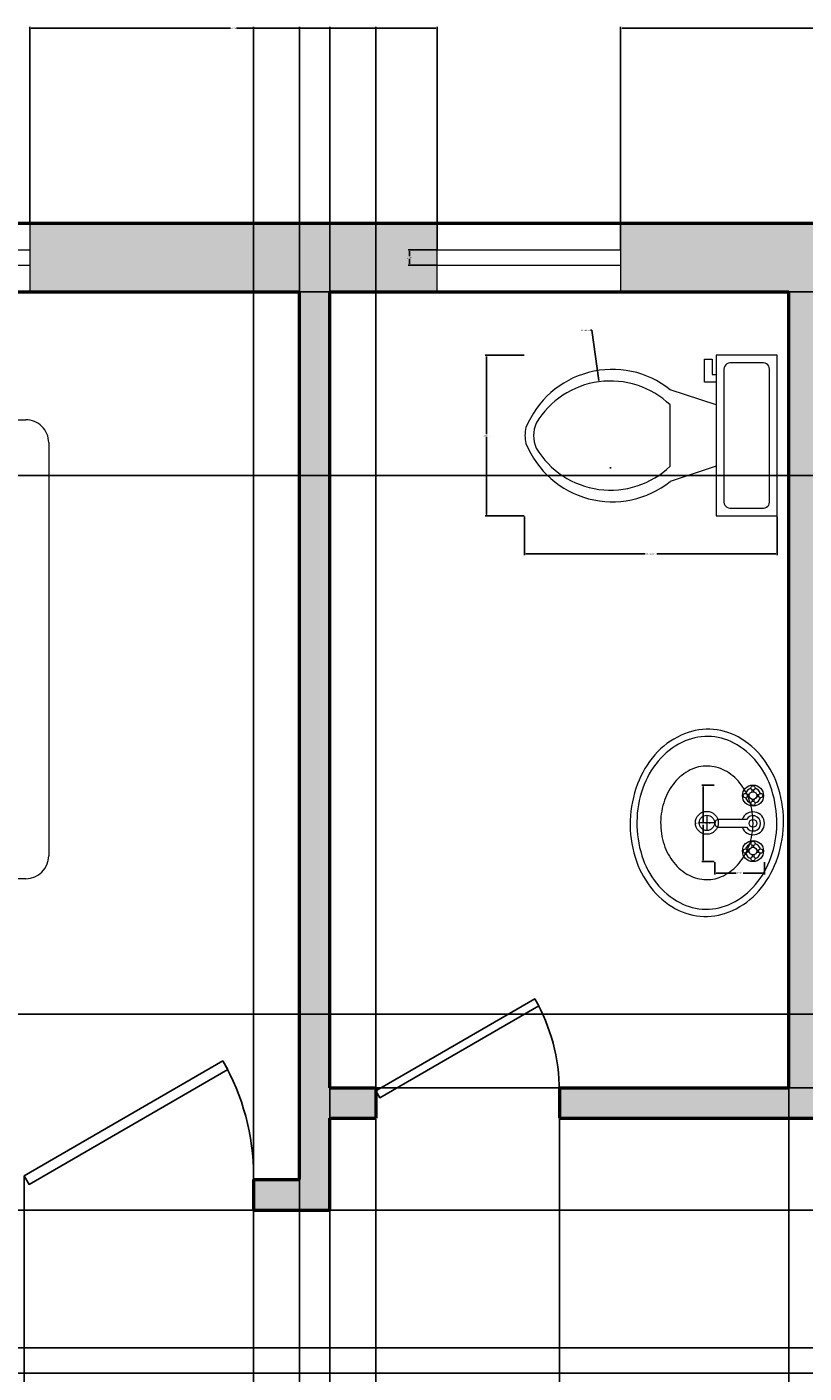
# Model space of a CAD drawing. Units: inches. Extents: x 3439 to 3988, y 1915 to 2284.
# Tile 3 of 7: x 3554 to 3656, y 2108 to 2284. Entities that reach past the tile are written whole.
import ezdxf

# ---------------------------------------------------------------- set-up
doc = ezdxf.new("R2010")
doc.units = ezdxf.units.IN
for name, color, linetype, lineweight in [('A-ANNO-DIMS', 2, 'Continuous', 18), ('A-DOOR', 3, 'Continuous', 25), ('A-FLOR-FIXT', 9, 'Continuous', 18), ('A-FURN', 9, 'Continuous', 18), ('A-GLAZ', 4, 'Continuous', 18), ('A-WALL', 7, 'Continuous', 50)]:
    doc.layers.add(name, color=color, linetype=linetype, lineweight=lineweight)
doc.layers.add('A-WALL-PATT', color=18, linetype='Continuous', lineweight=13, true_color=0x000000)
doc.styles.get("Standard").update_dxf_attribs({"font": 'arial.ttf'})
doc.dimstyles.get("Standard").update_dxf_attribs({"dimtxt": 0.18, "dimasz": 0.18, "dimexe": 0.18, "dimexo": 0.0625, "dimgap": 0.09, "dimtad": 0, "dimtih": 1, "dimtoh": 1, "dimdec": 4, "dimzin": 0, "dimdsep": 46, "dimtxsty": 'Standard', "dimcen": 0.09, "dimadec": 0, "dimazin": 0, "dimtfac": 1, "dimtdec": 4, "dimtofl": 0, "dimtmove": 0, "dimatfit": 3, "dimfxl": 1, "dimtolj": 1, "dimtzin": 0, "dimarcsym": 0})

# ---------------------------------------------------------------- blocks, each defined once
blk = doc.blocks.new('*U4')
for p, q in [((0, 0), (0, -6)), ((40, 0), (40, -6))]:
    blk.add_line(p, q)
blk.add_lwpolyline([(0, 0), (34.64, 20), (35.52, 18.48), (0.87, -1.52)], close=True)
blk.add_arc((0, 0), 40, 0, 30)
blk = doc.blocks.new('Sink - Oval top')
for p, q in [((-1, 0), (1, 0)), ((0, 1), (0, -1))]:
    blk.add_line(p, q)
for points in [[(-12.23, 0.39, 0.117634), (-11.46, -3.36, 0.104469), (-8.88, -6.8, 0.090016), (-5.08, -9.07, 0.08192), (-0.32, -10.02, 0.08192), (4.49, -9.38, 0.090016), (8.42, -7.36, 0.104469), (11.22, -4.09, 0.117634), (12.23, -0.39, 0.117634), (11.46, 3.36, 0.104469), (8.88, 6.8, 0.090016), (5.08, 9.07, 0.08192), (0.32, 10.02, 0.08192), (-4.49, 9.38, 0.090016), (-8.42, 7.36, 0.104469), (-11.22, 4.09, 0.117634)], [(-11.29, 0.16, 0.118622), (-10.52, -3.25, 0.104678), (-8.07, -6.36, 0.089562), (-4.54, -8.37, 0.081185), (-0.13, -9.15, 0.081185), (4.3, -8.49, 0.089562), (7.89, -6.58, 0.104678), (10.42, -3.55, 0.118622), (11.29, -0.16, 0.118622), (10.52, 3.25, 0.104678), (8.07, 6.36, 0.089562), (4.54, 8.37, 0.081185), (0.13, 9.15, 0.081185), (-4.3, 8.49, 0.089562), (-7.89, 6.58, 0.104678), (-10.42, 3.55, 0.118622)], [(-7.42, 0.08, 0.118283), (-6.91, -2.17, 0.104607), (-5.29, -4.21, 0.089718), (-2.97, -5.53, 0.081436), (-0.07, -6.04, 0.081436), (2.84, -5.59, 0.089718), (5.2, -4.33, 0.104607), (6.86, -2.32, 0.118283), (7.42, -0.08, 0.118283), (6.91, 2.17, 0.104607), (5.29, 4.21, 0.089718), (2.97, 5.53, 0.081436), (0.07, 6.04, 0.081436), (-2.84, 5.59, 0.089718), (-5.2, 4.33, 0.104607), (-6.86, 2.32, 0.118283)]]:
    blk.add_lwpolyline(points, format="xyb", close=True)
for radius in [1.5, 1]:
    blk.add_circle((0, 0), radius)
blk = doc.blocks.new('Faucet - Bathroom top')
for p, q in [((-4.107, 0.125), (-4.375, 0.125)), ((-3.75, 0.4788), (-3.75, 0.75)), ((-3.5, 0.482), (-3.5, 0.75)), ((-3.1461, 0.125), (-2.875, 0.125)), ((3.143, 0.125), (2.875, 0.125)), ((3.5, 0.4788), (3.5, 0.75)), ((3.75, 0.482), (3.75, 0.75)), ((4.1039, 0.125), (4.375, 0.125)), ((-4.1039, -0.125), (-4.375, -0.125)), ((-3.75, -0.4821), (-3.75, -0.75)), ((-3.5, -0.4789), (-3.5, -0.75)), ((-3.143, -0.125), (-2.875, -0.125)), ((-0.5, -0.8639), (-0.5, -4.5)), ((0.5, -4.5), (0.5, -0.8631)), ((3.1461, -0.125), (2.875, -0.125)), ((3.5, -0.4821), (3.5, -0.75)), ((3.75, -0.4789), (3.75, -0.75)), ((4.107, -0.125), (4.375, -0.125))]:
    blk.add_line(p, q)
for centre, radius in [((-3.625, 0), 1.375), ((-4.625, 0), 0.2795), ((-3.625, 0), 0.5), ((-3.625, 1), 0.2795), ((-2.625, 0), 0.2795), ((0, 0), 0.5), ((3.625, 0), 1.375), ((2.625, 0), 0.2795), ((3.625, 0), 0.5), ((3.625, 1), 0.2795), ((4.625, 0), 0.2795), ((-3.625, -1), 0.2795), ((3.625, -1), 0.2795)]:
    blk.add_circle(centre, radius)
for centre, radius, start, end in [((-3.625, 0), 1, 105.2407, 164.2093), ((-3.625, 0), 1, 16.44125, 74.07887), ((0, 0), 1.5, 289.6514, 250.3603), ((0, 0), 1, 300.3431, 239.7554), ((3.625, 0), 1, 106.12, 164.0884), ((3.625, 0), 1, 16.23422, 73.90469), ((-3.625, 0), 1, 196.2342, 253.9047), ((-3.625, 0), 1, 286.12, 344.0884), ((3.625, 0), 1, 196.4413, 254.0789), ((3.625, 0), 1, 285.2407, 344.2093), ((0, -4.5), 0.5, 180, 0)]:
    blk.add_arc(centre, radius, start, end)
blk = doc.blocks.new('Bed - Queen')
for p, q in [((3, 0), (56.99999, 0)), ((10.99999, -1.2), (25.79998, -1.2)), ((34.19999, -1.2), (48.99999, -1.2)), ((0, -77.00003), (0, -3)), ((59.99999, -3), (59.99999, -77.00003)), ((7.99999, -14.4), (7.99999, -4.2)), ((28.79998, -4.2), (28.79998, -14.4)), ((31.19999, -14.4), (31.19999, -4.2)), ((51.99999, -4.2), (51.99999, -13.4)), ((0, -14.4), (44.8, -14.4)), ((59.99999, -29.6), (44.8, -14.4)), ((44.8, -14.4), (44.8, -26.6)), ((44.8, -16.8), (0, -16.8)), ((48.99999, -16.4), (46.79936, -16.4)), ((47.8, -29.6), (59.99999, -29.6)), ((56.99999, -80.00003), (3, -80.00003))]:
    blk.add_line(p, q)
for centre, start, end in [((3, -3), 90, 180), ((56.99999, -3), 0, 90), ((10.99999, -4.2), 90, 180), ((25.79998, -4.2), 0, 90), ((34.19999, -4.2), 90, 180), ((48.99999, -4.2), 0, 90), ((48.99999, -13.4), 270, 0), ((47.8, -26.6), 180, 270), ((3, -77.00003), 180, 270), ((56.99999, -77.00003), 270, 0)]:
    blk.add_arc(centre, 3, start, end)
blk = doc.blocks.new('Toilet - top')
for p, q in [((9.5, -6), (9.5, -2)), ((-10, -8.5), (-8, -8.5)), ((-10, -9.5), (-10, -8.5)), ((-8, -8.5), (-8, -8)), ((-7, -8), (-7, -9.5)), ((-4, -8), (-6, -14)), ((4, -8), (6, -14)), ((-7, -9.5), (-10, -9.5)), ((4, -14), (-4, -14))]:
    blk.add_line(p, q)
blk.add_lwpolyline([(10.5, -8), (10.5, 0), (-10.5, 0), (-10.5, -8)], close=True)
for points in [[(8.5, -1), (-8.5, -1)], [(-9.5, -2), (-9.5, -6)], [(-8.5, -7), (8.5, -7)]]:
    blk.add_lwpolyline(points)
for centre, radius, start, end in [((-8.62, -1.88), 0.884, 81.8699, 188.1301), ((8.62, -1.88), 0.884, 351.8699, 98.1301), ((-8.62, -6.12), 0.884, 171.8699, 278.1301), ((8.62, -6.12), 0.884, 261.8699, 8.1301), ((3.52, -21.58), 12.17, 141.4691, 247.9714), ((4.2, -21.82), 11.33, 136.3677, 238.9468), ((-3.52, -21.58), 12.17, 292.0284, 38.5307), ((-4.2, -21.82), 11.33, 301.053, 43.6321), ((0, -27.88), 4, 245.7318, 294.2682), ((0, -29), 4, 254.8605, 285.1395)]:
    blk.add_arc(centre, radius, start, end)
blk = doc.blocks.new('WINDOW-GLASS-48IN')
for p, q in [((0, 2), (48, 2)), ((0, 0), (48, 0))]:
    blk.add_line(p, q)
blk = doc.blocks.new('WINDOW-GLASS-24IN')
for p, q in [((0, 2), (24, 2)), ((0, 0), (24, 0))]:
    blk.add_line(p, q)
blk = doc.blocks.new('*D21')
at = {"layer": 'A-ANNO-DIMS', "color": 0, "lineweight": -2, "transparency": 16777216}
for p, q in [((3607.59, 2254.92), (3607.59, 2258.64)), ((3607.77, 2258.46), (3618.48, 2258.46)), ((3631.41, 2258.46), (3620.71, 2258.46)), ((3631.59, 2254.92), (3631.59, 2258.64))]:
    blk.add_line(p, q, dxfattribs=at)
at = {"layer": 'A-ANNO-DIMS', "color": 0, "transparency": 16777216}
for points in [[(3607.77, 2258.49), (3607.77, 2258.43), (3607.59, 2258.46)], [(3631.41, 2258.49), (3631.41, 2258.43), (3631.59, 2258.46)]]:
    blk.add_solid(points, dxfattribs=at)
at = {"layer": 'Defpoints', "color": 0, "transparency": 16777216}
for p in [(3631.59, 2258.46), (3607.59, 2254.86), (3631.59, 2254.86)]:
    blk.add_point(p, dxfattribs=at)
at = {"layer": 'A-ANNO-DIMS', "color": 0, "transparency": 16777216, "insert": (3619.59, 2258.46), "char_height": 0.18, "attachment_point": 5}
blk.add_mtext('\\A1;WINDOW 24 TYP.', dxfattribs=at)
blk = doc.blocks.new('*D22')
at = {"layer": 'A-ANNO-DIMS', "color": 0, "lineweight": -2, "transparency": 16777216}
for p, q in [((3607.53, 2254.86), (3603.81, 2254.86)), ((3603.99, 2254.68), (3603.99, 2254.04)), ((3607.53, 2252.86), (3603.81, 2252.86)), ((3603.99, 2253.04), (3603.99, 2253.68))]:
    blk.add_line(p, q, dxfattribs=at)
at = {"layer": 'A-ANNO-DIMS', "color": 0, "transparency": 16777216}
for points in [[(3603.96, 2254.68), (3604.02, 2254.68), (3603.99, 2254.86)], [(3603.96, 2253.04), (3604.02, 2253.04), (3603.99, 2252.86)]]:
    blk.add_solid(points, dxfattribs=at)
at = {"layer": 'Defpoints', "color": 0, "transparency": 16777216}
for p in [(3603.99, 2254.86), (3607.59, 2254.86), (3607.59, 2252.86)]:
    blk.add_point(p, dxfattribs=at)
at = {"layer": 'A-ANNO-DIMS', "color": 0, "transparency": 16777216, "insert": (3603.99, 2253.86), "char_height": 0.18, "attachment_point": 5}
blk.add_mtext('\\A1;2 TYP.', dxfattribs=at)
blk = doc.blocks.new('*D31')
at = {"layer": 'A-ANNO-DIMS', "color": 0, "lineweight": -2, "transparency": 16777216}
for p, q in [((3619.03, 2220.03), (3619.03, 2214.95)), ((3652.08, 2220.03), (3652.08, 2214.95)), ((3619.21, 2215.13), (3634.78, 2215.13)), ((3651.9, 2215.13), (3636.33, 2215.13))]:
    blk.add_line(p, q, dxfattribs=at)
at = {"layer": 'A-ANNO-DIMS', "color": 0, "transparency": 16777216}
for points in [[(3619.21, 2215.16), (3619.21, 2215.1), (3619.03, 2215.13)], [(3651.9, 2215.16), (3651.9, 2215.1), (3652.08, 2215.13)]]:
    blk.add_solid(points, dxfattribs=at)
at = {"layer": 'Defpoints', "color": 0, "transparency": 16777216}
for p in [(3619.03, 2220.09), (3652.08, 2220.09), (3652.08, 2215.13)]:
    blk.add_point(p, dxfattribs=at)
at = {"layer": 'A-ANNO-DIMS', "color": 0, "transparency": 16777216, "insert": (3635.55, 2215.13), "char_height": 0.18, "attachment_point": 5}
blk.add_mtext('\\A1;WC 33 TYP.', dxfattribs=at)
blk = doc.blocks.new('*D32')
at = {"layer": 'A-ANNO-DIMS', "color": 0, "lineweight": -2, "transparency": 16777216}
for p, q in [((3618.97, 2241.09), (3613.89, 2241.09)), ((3614.07, 2240.91), (3614.07, 2230.77)), ((3614.07, 2220.27), (3614.07, 2230.41)), ((3618.97, 2220.09), (3613.89, 2220.09))]:
    blk.add_line(p, q, dxfattribs=at)
at = {"layer": 'A-ANNO-DIMS', "color": 0, "transparency": 16777216}
for points in [[(3614.04, 2240.91), (3614.1, 2240.91), (3614.07, 2241.09)], [(3614.04, 2220.27), (3614.1, 2220.27), (3614.07, 2220.09)]]:
    blk.add_solid(points, dxfattribs=at)
at = {"layer": 'Defpoints', "color": 0, "transparency": 16777216}
for p in [(3619.03, 2241.09), (3614.07, 2220.09), (3619.03, 2220.09)]:
    blk.add_point(p, dxfattribs=at)
at = {"layer": 'A-ANNO-DIMS', "color": 0, "transparency": 16777216, "insert": (3614.07, 2230.59), "char_height": 0.18, "attachment_point": 5}
blk.add_mtext('\\A1;21 TYP.', dxfattribs=at)
blk = doc.blocks.new('*D35')
at = {"layer": 'A-ANNO-DIMS', "color": 0, "lineweight": -2, "transparency": 16777216}
for p, q in [((3643.84, 2184.91), (3642.22, 2184.91)), ((3642.4, 2184.73), (3642.4, 2180.1)), ((3642.4, 2175.09), (3642.4, 2179.73)), ((3643.84, 2174.91), (3642.22, 2174.91))]:
    blk.add_line(p, q, dxfattribs=at)
at = {"layer": 'A-ANNO-DIMS', "color": 0, "transparency": 16777216}
for points in [[(3642.37, 2184.73), (3642.43, 2184.73), (3642.4, 2184.91)], [(3642.37, 2175.09), (3642.43, 2175.09), (3642.4, 2174.91)]]:
    blk.add_solid(points, dxfattribs=at)
at = {"layer": 'Defpoints', "color": 0, "transparency": 16777216}
for p in [(3643.9, 2184.91), (3642.4, 2174.91), (3643.9, 2174.91)]:
    blk.add_point(p, dxfattribs=at)
at = {"layer": 'A-ANNO-DIMS', "color": 0, "transparency": 16777216, "insert": (3642.4, 2179.91), "char_height": 0.18, "attachment_point": 5}
blk.add_mtext('\\A1;BASIN TAP 10 TYP.', dxfattribs=at)
blk = doc.blocks.new('*D36')
at = {"layer": 'A-ANNO-DIMS', "color": 0, "lineweight": -2, "transparency": 16777216}
for p, q in [((3643.9, 2174.85), (3643.9, 2173.23)), ((3650.4, 2174.85), (3650.4, 2173.23)), ((3644.08, 2173.41), (3646.69, 2173.41)), ((3650.22, 2173.41), (3647.61, 2173.41))]:
    blk.add_line(p, q, dxfattribs=at)
at = {"layer": 'A-ANNO-DIMS', "color": 0, "transparency": 16777216}
for points in [[(3644.08, 2173.44), (3644.08, 2173.38), (3643.9, 2173.41)], [(3650.22, 2173.44), (3650.22, 2173.38), (3650.4, 2173.41)]]:
    blk.add_solid(points, dxfattribs=at)
at = {"layer": 'Defpoints', "color": 0, "transparency": 16777216}
for p in [(3643.9, 2174.91), (3650.4, 2174.91), (3650.4, 2173.41)]:
    blk.add_point(p, dxfattribs=at)
at = {"layer": 'A-ANNO-DIMS', "color": 0, "transparency": 16777216, "insert": (3647.15, 2173.41), "char_height": 0.18, "attachment_point": 5}
blk.add_mtext('\\A1;7 TYP.', dxfattribs=at)
blk = doc.blocks.new('*D47')
at = {"layer": 'A-ANNO-DIMS', "color": 0, "lineweight": -2, "transparency": 16777216}
for p, q in [((3473.58, 2249.3), (3473.58, 1915.13)), ((3589.58, 2249.3), (3589.58, 1915.13)), ((3473.76, 1915.31), (3531.3, 1915.31)), ((3589.4, 1915.31), (3531.86, 1915.31))]:
    blk.add_line(p, q, dxfattribs=at)
at = {"layer": 'A-ANNO-DIMS', "color": 0, "transparency": 16777216}
for points in [[(3473.76, 1915.34), (3473.76, 1915.28), (3473.58, 1915.31)], [(3589.4, 1915.34), (3589.4, 1915.28), (3589.58, 1915.31)]]:
    blk.add_solid(points, dxfattribs=at)
at = {"layer": 'Defpoints', "color": 0, "transparency": 16777216}
for p in [(3473.58, 2249.36), (3589.58, 2249.36), (3589.58, 1915.31)]:
    blk.add_point(p, dxfattribs=at)
at = {"layer": 'A-ANNO-DIMS', "color": 0, "transparency": 16777216, "insert": (3531.58, 1915.31), "char_height": 0.18, "attachment_point": 5}
blk.add_mtext('\\A1;116', dxfattribs=at)
blk = doc.blocks.new('*D48')
at = {"layer": 'A-ANNO-DIMS', "color": 0, "lineweight": -2, "transparency": 16777216}
for p, q in [((3593.58, 2249.3), (3593.58, 1915.13)), ((3653.58, 2249.3), (3653.58, 1915.13)), ((3593.76, 1915.31), (3623.36, 1915.31)), ((3653.4, 1915.31), (3623.8, 1915.31))]:
    blk.add_line(p, q, dxfattribs=at)
at = {"layer": 'A-ANNO-DIMS', "color": 0, "transparency": 16777216}
for points in [[(3593.76, 1915.34), (3593.76, 1915.28), (3593.58, 1915.31)], [(3653.4, 1915.34), (3653.4, 1915.28), (3653.58, 1915.31)]]:
    blk.add_solid(points, dxfattribs=at)
at = {"layer": 'Defpoints', "color": 0, "transparency": 16777216}
for p in [(3593.58, 2249.36), (3653.58, 2249.36), (3653.58, 1915.31)]:
    blk.add_point(p, dxfattribs=at)
at = {"layer": 'A-ANNO-DIMS', "color": 0, "transparency": 16777216, "insert": (3623.58, 1915.31), "char_height": 0.18, "attachment_point": 5}
blk.add_mtext('\\A1;60', dxfattribs=at)
blk = doc.blocks.new('*D64')
at = {"layer": 'A-ANNO-DIMS', "color": 0, "lineweight": -2, "transparency": 16777216}
for p, q in [((3593.64, 2249.36), (3987.81, 2249.36)), ((3987.63, 2249.18), (3987.63, 2197.54)), ((3987.63, 2145.54), (3987.63, 2197.18)), ((3593.64, 2145.36), (3987.81, 2145.36))]:
    blk.add_line(p, q, dxfattribs=at)
at = {"layer": 'A-ANNO-DIMS', "color": 0, "transparency": 16777216}
for points in [[(3987.6, 2249.18), (3987.66, 2249.18), (3987.63, 2249.36)], [(3987.6, 2145.54), (3987.66, 2145.54), (3987.63, 2145.36)]]:
    blk.add_solid(points, dxfattribs=at)
at = {"layer": 'Defpoints', "color": 0, "transparency": 16777216}
for p in [(3593.58, 2249.36), (3987.63, 2249.36), (3593.58, 2145.36)]:
    blk.add_point(p, dxfattribs=at)
at = {"layer": 'A-ANNO-DIMS', "color": 0, "transparency": 16777216, "insert": (3987.63, 2197.36), "char_height": 0.18, "attachment_point": 5}
blk.add_mtext('\\A1;104', dxfattribs=at)
blk = doc.blocks.new('*D67')
at = {"layer": 'A-ANNO-DIMS', "color": 0, "lineweight": -2, "transparency": 16777216}
for p, q in [((3554.32, 2258.42), (3554.32, 2284)), ((3554.5, 2283.82), (3580.56, 2283.82)), ((3607.41, 2283.82), (3581.35, 2283.82)), ((3607.59, 2258.42), (3607.59, 2284))]:
    blk.add_line(p, q, dxfattribs=at)
at = {"layer": 'A-ANNO-DIMS', "color": 0, "transparency": 16777216}
for points in [[(3554.5, 2283.85), (3554.5, 2283.79), (3554.32, 2283.82)], [(3607.41, 2283.85), (3607.41, 2283.79), (3607.59, 2283.82)]]:
    blk.add_solid(points, dxfattribs=at)
at = {"layer": 'Defpoints', "color": 0, "transparency": 16777216}
for p in [(3607.59, 2283.82), (3554.32, 2258.36), (3607.59, 2258.36)]:
    blk.add_point(p, dxfattribs=at)
at = {"layer": 'A-ANNO-DIMS', "color": 0, "transparency": 16777216, "insert": (3580.96, 2283.82), "char_height": 0.18, "attachment_point": 5}
blk.add_mtext('\\A1;53.28', dxfattribs=at)
blk = doc.blocks.new('*D68')
at = {"layer": 'A-ANNO-DIMS', "color": 0, "lineweight": -2, "transparency": 16777216}
for p, q in [((3631.59, 2258.42), (3631.59, 2284)), ((3631.77, 2283.82), (3661.12, 2283.82)), ((3691.23, 2283.82), (3661.88, 2283.82)), ((3691.41, 2258.42), (3691.41, 2284))]:
    blk.add_line(p, q, dxfattribs=at)
at = {"layer": 'A-ANNO-DIMS', "color": 0, "transparency": 16777216}
for points in [[(3631.77, 2283.85), (3631.77, 2283.79), (3631.59, 2283.82)], [(3691.23, 2283.85), (3691.23, 2283.79), (3691.41, 2283.82)]]:
    blk.add_solid(points, dxfattribs=at)
at = {"layer": 'Defpoints', "color": 0, "transparency": 16777216}
for p in [(3691.41, 2283.82), (3631.59, 2258.36), (3691.41, 2258.36)]:
    blk.add_point(p, dxfattribs=at)
at = {"layer": 'A-ANNO-DIMS', "color": 0, "transparency": 16777216, "insert": (3661.5, 2283.82), "char_height": 0.18, "attachment_point": 5}
blk.add_mtext('\\A1;59.81', dxfattribs=at)
blk = doc.blocks.new('*D77')
at = {"layer": 'A-ANNO-DIMS', "color": 0, "lineweight": -2, "transparency": 16777216}
for p, q in [((3473.64, 2129.36), (3987.81, 2129.36)), ((3987.63, 2129.18), (3987.63, 2118.9)), ((3987.63, 2108.25), (3987.63, 2118.53)), ((3473.64, 2108.07), (3987.81, 2108.07))]:
    blk.add_line(p, q, dxfattribs=at)
at = {"layer": 'A-ANNO-DIMS', "color": 0, "transparency": 16777216}
for points in [[(3987.6, 2129.18), (3987.66, 2129.18), (3987.63, 2129.36)], [(3987.6, 2108.25), (3987.66, 2108.25), (3987.63, 2108.07)]]:
    blk.add_solid(points, dxfattribs=at)
at = {"layer": 'Defpoints', "color": 0, "transparency": 16777216}
for p in [(3473.58, 2129.36), (3987.63, 2129.36), (3473.58, 2108.07)]:
    blk.add_point(p, dxfattribs=at)
at = {"layer": 'A-ANNO-DIMS', "color": 0, "transparency": 16777216, "insert": (3987.63, 2118.71), "char_height": 0.18, "attachment_point": 5}
blk.add_mtext('\\A1;21.295', dxfattribs=at)
blk = doc.blocks.new('*D78')
at = {"layer": 'A-ANNO-DIMS', "color": 0, "lineweight": -2, "transparency": 16777216}
for p, q in [((3553.58, 2129.3), (3553.58, 1915.13)), ((3583.58, 2129.3), (3583.58, 1915.13)), ((3553.76, 1915.31), (3568.36, 1915.31)), ((3583.4, 1915.31), (3568.8, 1915.31))]:
    blk.add_line(p, q, dxfattribs=at)
at = {"layer": 'A-ANNO-DIMS', "color": 0, "transparency": 16777216}
for points in [[(3553.76, 1915.34), (3553.76, 1915.28), (3553.58, 1915.31)], [(3583.4, 1915.34), (3583.4, 1915.28), (3583.58, 1915.31)]]:
    blk.add_solid(points, dxfattribs=at)
at = {"layer": 'Defpoints', "color": 0, "transparency": 16777216}
for p in [(3553.58, 2129.36), (3583.58, 2129.36), (3583.58, 1915.31)]:
    blk.add_point(p, dxfattribs=at)
at = {"layer": 'A-ANNO-DIMS', "color": 0, "transparency": 16777216, "insert": (3568.58, 1915.31), "char_height": 0.18, "attachment_point": 5}
blk.add_mtext('\\A1;30', dxfattribs=at)
blk = doc.blocks.new('*D79')
at = {"layer": 'A-ANNO-DIMS', "color": 0, "lineweight": -2, "transparency": 16777216}
for p, q in [((3583.58, 2133.42), (3583.58, 2284)), ((3583.76, 2283.82), (3586.43, 2283.82)), ((3589.4, 2283.82), (3586.73, 2283.82)), ((3589.58, 2133.42), (3589.58, 2284))]:
    blk.add_line(p, q, dxfattribs=at)
at = {"layer": 'A-ANNO-DIMS', "color": 0, "transparency": 16777216}
for points in [[(3583.76, 2283.85), (3583.76, 2283.79), (3583.58, 2283.82)], [(3589.4, 2283.85), (3589.4, 2283.79), (3589.58, 2283.82)]]:
    blk.add_solid(points, dxfattribs=at)
at = {"layer": 'Defpoints', "color": 0, "transparency": 16777216}
for p in [(3589.58, 2283.82), (3583.58, 2133.36), (3589.58, 2133.36)]:
    blk.add_point(p, dxfattribs=at)
at = {"layer": 'A-ANNO-DIMS', "color": 0, "transparency": 16777216, "insert": (3586.58, 2283.82), "char_height": 0.18, "attachment_point": 5}
blk.add_mtext('\\A1;6', dxfattribs=at)
blk = doc.blocks.new('*D80')
at = {"layer": 'A-ANNO-DIMS', "color": 0, "lineweight": -2, "transparency": 16777216}
for p, q in [((3599.58, 2141.3), (3599.58, 1915.13)), ((3623.58, 2141.3), (3623.58, 1915.13)), ((3599.76, 1915.31), (3611.36, 1915.31)), ((3623.4, 1915.31), (3611.8, 1915.31))]:
    blk.add_line(p, q, dxfattribs=at)
at = {"layer": 'A-ANNO-DIMS', "color": 0, "transparency": 16777216}
for points in [[(3599.76, 1915.34), (3599.76, 1915.28), (3599.58, 1915.31)], [(3623.4, 1915.34), (3623.4, 1915.28), (3623.58, 1915.31)]]:
    blk.add_solid(points, dxfattribs=at)
at = {"layer": 'Defpoints', "color": 0, "transparency": 16777216}
for p in [(3599.58, 2141.36), (3623.58, 2141.36), (3623.58, 1915.31)]:
    blk.add_point(p, dxfattribs=at)
at = {"layer": 'A-ANNO-DIMS', "color": 0, "transparency": 16777216, "insert": (3611.58, 1915.31), "char_height": 0.18, "attachment_point": 5}
blk.add_mtext('\\A1;24', dxfattribs=at)
blk = doc.blocks.new('*D81')
at = {"layer": 'A-ANNO-DIMS', "color": 0, "lineweight": -2, "transparency": 16777216}
for p, q in [((3593.58, 2145.42), (3593.58, 2284)), ((3593.76, 2283.82), (3596.43, 2283.82)), ((3599.4, 2283.82), (3596.73, 2283.82)), ((3599.58, 2145.42), (3599.58, 2284))]:
    blk.add_line(p, q, dxfattribs=at)
at = {"layer": 'A-ANNO-DIMS', "color": 0, "transparency": 16777216}
for points in [[(3593.76, 2283.85), (3593.76, 2283.79), (3593.58, 2283.82)], [(3599.4, 2283.85), (3599.4, 2283.79), (3599.58, 2283.82)]]:
    blk.add_solid(points, dxfattribs=at)
at = {"layer": 'Defpoints', "color": 0, "transparency": 16777216}
for p in [(3599.58, 2283.82), (3593.58, 2145.36), (3599.58, 2145.36)]:
    blk.add_point(p, dxfattribs=at)
at = {"layer": 'A-ANNO-DIMS', "color": 0, "transparency": 16777216, "insert": (3596.58, 2283.82), "char_height": 0.18, "attachment_point": 5}
blk.add_mtext('\\A1;6', dxfattribs=at)
blk = doc.blocks.new('*D82')
at = {"layer": 'A-ANNO-DIMS', "color": 0, "lineweight": -2, "transparency": 16777216}
for p, q in [((3537.64, 2129.36), (3987.81, 2129.36)), ((3987.63, 2129.18), (3987.63, 2120.54)), ((3987.63, 2111.54), (3987.63, 2120.18)), ((3537.64, 2111.36), (3987.81, 2111.36))]:
    blk.add_line(p, q, dxfattribs=at)
at = {"layer": 'A-ANNO-DIMS', "color": 0, "transparency": 16777216}
for points in [[(3987.6, 2129.18), (3987.66, 2129.18), (3987.63, 2129.36)], [(3987.6, 2111.54), (3987.66, 2111.54), (3987.63, 2111.36)]]:
    blk.add_solid(points, dxfattribs=at)
at = {"layer": 'Defpoints', "color": 0, "transparency": 16777216}
for p in [(3537.58, 2129.36), (3987.63, 2129.36), (3537.58, 2111.36)]:
    blk.add_point(p, dxfattribs=at)
at = {"layer": 'A-ANNO-DIMS', "color": 0, "transparency": 16777216, "insert": (3987.63, 2120.36), "char_height": 0.18, "attachment_point": 5}
blk.add_mtext('\\A1;18', dxfattribs=at)
blk = doc.blocks.new('*D83')
at = {"layer": 'A-ANNO-DIMS', "color": 0, "lineweight": -2, "transparency": 16777216}
for p, q in [((3537.64, 2111.36), (3987.81, 2111.36)), ((3987.63, 2111.18), (3987.63, 2099.54)), ((3987.63, 2087.54), (3987.63, 2099.18)), ((3537.64, 2087.36), (3987.81, 2087.36))]:
    blk.add_line(p, q, dxfattribs=at)
at = {"layer": 'A-ANNO-DIMS', "color": 0, "transparency": 16777216}
for points in [[(3987.6, 2111.18), (3987.66, 2111.18), (3987.63, 2111.36)], [(3987.6, 2087.54), (3987.66, 2087.54), (3987.63, 2087.36)]]:
    blk.add_solid(points, dxfattribs=at)
at = {"layer": 'Defpoints', "color": 0, "transparency": 16777216}
for p in [(3537.58, 2111.36), (3987.63, 2111.36), (3537.58, 2087.36)]:
    blk.add_point(p, dxfattribs=at)
at = {"layer": 'A-ANNO-DIMS', "color": 0, "transparency": 16777216, "insert": (3987.63, 2099.36), "char_height": 0.18, "attachment_point": 5}
blk.add_mtext('\\A1;24', dxfattribs=at)
blk = doc.blocks.new('*D96')
at = {"layer": 'A-ANNO-DIMS', "color": 0, "lineweight": -2, "transparency": 16777216}
for p, q in [((3793.87, 2249.36), (3439.35, 2249.36)), ((3439.53, 2249.18), (3439.53, 2237.54)), ((3439.53, 2225.54), (3439.53, 2237.18)), ((3769.87, 2225.36), (3439.35, 2225.36))]:
    blk.add_line(p, q, dxfattribs=at)
at = {"layer": 'A-ANNO-DIMS', "color": 0, "transparency": 16777216}
for points in [[(3439.5, 2249.18), (3439.56, 2249.18), (3439.53, 2249.36)], [(3439.5, 2225.54), (3439.56, 2225.54), (3439.53, 2225.36)]]:
    blk.add_solid(points, dxfattribs=at)
at = {"layer": 'Defpoints', "color": 0, "transparency": 16777216}
for p in [(3439.53, 2249.36), (3793.93, 2249.36), (3769.93, 2225.36)]:
    blk.add_point(p, dxfattribs=at)
at = {"layer": 'A-ANNO-DIMS', "color": 0, "transparency": 16777216, "insert": (3439.53, 2237.36), "char_height": 0.18, "attachment_point": 5}
blk.add_mtext('\\A1;24', dxfattribs=at)
blk = doc.blocks.new('*D98')
at = {"layer": 'A-ANNO-DIMS', "color": 0, "lineweight": -2, "transparency": 16777216}
for p, q in [((3889.52, 2154.99), (3439.35, 2154.99)), ((3439.53, 2154.81), (3439.53, 2142.36)), ((3439.53, 2129.54), (3439.53, 2141.99)), ((3889.52, 2129.36), (3439.35, 2129.36))]:
    blk.add_line(p, q, dxfattribs=at)
at = {"layer": 'A-ANNO-DIMS', "color": 0, "transparency": 16777216}
for points in [[(3439.5, 2154.81), (3439.56, 2154.81), (3439.53, 2154.99)], [(3439.5, 2129.54), (3439.56, 2129.54), (3439.53, 2129.36)]]:
    blk.add_solid(points, dxfattribs=at)
at = {"layer": 'Defpoints', "color": 0, "transparency": 16777216}
for p in [(3889.58, 2154.99), (3439.53, 2129.36), (3889.58, 2129.36)]:
    blk.add_point(p, dxfattribs=at)
at = {"layer": 'A-ANNO-DIMS', "color": 0, "transparency": 16777216, "insert": (3439.53, 2142.18), "char_height": 0.18, "attachment_point": 5}
blk.add_mtext('\\A1;25.63', dxfattribs=at)
blk = doc.blocks.new('*D104')
at = {"layer": 'A-ANNO-DIMS', "color": 0, "lineweight": -2, "transparency": 16777216}
for p, q in [((3627.66, 2244.36), (3627.84, 2244.36)), ((3627.84, 2244.36), (3628.73, 2237.8)), ((3630.17, 2226.39), (3630.35, 2226.39)), ((3630.26, 2226.3), (3630.26, 2226.48))]:
    blk.add_line(p, q, dxfattribs=at)
at = {"layer": 'A-ANNO-DIMS', "color": 0, "transparency": 16777216}
blk.add_solid([(3628.76, 2237.8), (3628.7, 2237.79), (3628.75, 2237.62)], dxfattribs=at)
at = {"layer": 'Defpoints', "color": 0, "transparency": 16777216}
for p in [(3628.75, 2237.62), (3630.26, 2226.39)]:
    blk.add_point(p, dxfattribs=at)
at = {"layer": 'A-ANNO-DIMS', "color": 0, "transparency": 16777216, "insert": (3626.99, 2244.36), "char_height": 0.18, "attachment_point": 5}
blk.add_mtext('\\A1;6X R11.33', dxfattribs=at)

msp = doc.modelspace()

# ---------------------------------------------------------------- hatches: boundary and pattern name
at = {"layer": 'A-WALL-PATT'}
h = msp.add_hatch(color=256, dxfattribs=at)
h.dxf.hatch_style = 1
h.paths.add_polyline_path([(3607.5949, 2258.3617), (3554.3179, 2258.3617), (3554.3179, 2249.3617), (3589.5815, 2249.3617), (3589.5815, 2133.3617), (3583.5815, 2133.3617), (3583.5815, 2129.3617), (3593.5815, 2129.3617), (3593.5815, 2141.3617), (3599.5815, 2141.3617), (3599.5815, 2144.9617), (3599.5815, 2145.3617), (3593.5815, 2145.3617), (3593.5815, 2249.3617), (3607.5949, 2249.3617)])
h = msp.add_hatch(color=256, dxfattribs=at)
h.dxf.hatch_style = 1
h.paths.add_polyline_path([(3691.4053, 2258.3617), (3631.5949, 2258.3617), (3631.5949, 2249.3617), (3653.5815, 2249.3617), (3653.5815, 2145.3617), (3623.5815, 2145.3617), (3623.5815, 2141.3617), (3657.5815, 2141.3617), (3657.5815, 2249.3617), (3691.4053, 2249.3617)])

# ---------------------------------------------------------------- linework, layer by layer
at = {"layer": 'A-GLAZ'}
for points in [[(3554.3179, 2258.3617), (3554.3179, 2249.3617)], [(3607.5949, 2249.3617), (3607.5949, 2258.3617)], [(3631.5949, 2258.3617), (3631.5949, 2249.3617)]]:
    msp.add_lwpolyline(points, dxfattribs=at)
at = {"layer": 'A-WALL'}
for p, q in [((3473.5815, 2249.3617), (3589.5815, 2249.3617)), ((3589.5815, 2133.3617), (3589.5815, 2249.3617)), ((3593.5815, 2249.3617), (3653.5815, 2249.3617)), ((3593.5815, 2145.3617), (3593.5815, 2249.3617)), ((3653.5815, 2145.3617), (3653.5815, 2249.3617)), ((3593.5815, 2145.3617), (3599.5815, 2145.3617)), ((3599.5815, 2145.3617), (3599.5815, 2141.3617)), ((3623.5815, 2145.3617), (3623.5815, 2141.3617)), ((3623.5815, 2145.3617), (3653.5815, 2145.3617)), ((3593.5815, 2129.3617), (3593.5815, 2141.3617)), ((3593.5815, 2129.3617), (3593.5815, 2141.3617)), ((3593.5815, 2141.3617), (3599.5815, 2141.3617)), ((3623.5815, 2141.3617), (3657.5815, 2141.3617)), ((3583.5815, 2133.3617), (3583.5815, 2129.3617)), ((3583.5815, 2133.3617), (3589.5815, 2133.3617)), ((3583.5815, 2129.3617), (3593.5815, 2129.3617))]:
    msp.add_line(p, q, dxfattribs=at)
msp.add_lwpolyline([(3719.5815, 1940.3617), (3464.5815, 1940.3617), (3464.5815, 2258.3617), (3803.9319, 2258.3617)], dxfattribs=at)

# ---------------------------------------------------------------- block references
at = {"layer": 'A-DOOR'}
for p, xscale, yscale, zscale in [((3599.5815, 2144.9617), 0.6000000000000001, 0.6000000000000001, 0.6000000000000001), ((3553.5815, 2133.8617), 0.75, 0.75, 0.75)]:
    msp.add_blockref('*U4', p, dxfattribs=dict(at, xscale=xscale, yscale=yscale, zscale=zscale))
at = {"layer": 'A-FLOR-FIXT', "rotation": 270}
for name, p in [('Toilet - top', (3652.0766, 2230.5918)), ('Sink - Oval top', (3642.8642, 2179.98)), ('Faucet - Bathroom top', (3648.901, 2179.9124))]:
    msp.add_blockref(name, p, dxfattribs=at)
at = {"layer": 'A-FURN', "rotation": 89.99999999999999}
msp.add_blockref('Bed - Queen', (3476.798, 2172.669), dxfattribs=at)
at = {"layer": 'A-GLAZ'}
for name, p in [('WINDOW-GLASS-48IN', (3506.3179, 2252.8617)), ('WINDOW-GLASS-24IN', (3607.5949, 2252.8617))]:
    msp.add_blockref(name, p, dxfattribs=at)

# ---------------------------------------------------------------- dimensions: what is measured, and where the dimension line sits
at = {"layer": 'A-ANNO-DIMS'}
for base, p1, p2, override, picture, middle in [((3607.5949, 2283.8228), (3554.3179, 2258.3617), (3607.5949, 2258.3617), {"dimdec": 2, "dimlfac": 1, "dimrnd": 0, "dimzin": 0, "dimdsep": 46, "dimlunit": 2}, '*D67', (3580.9564, 2283.8228)), ((3589.5815, 2283.8228), (3583.5815, 2133.3617), (3589.5815, 2133.3617), {"dimdec": 0, "dimlfac": 1, "dimrnd": 0, "dimzin": 0, "dimdsep": 46, "dimlunit": 2}, '*D79', (3586.5815, 2283.8228)), ((3599.5815, 2283.8228), (3593.5815, 2145.3617), (3599.5815, 2145.3617), {"dimdec": 0, "dimlfac": 1, "dimrnd": 0, "dimzin": 0, "dimdsep": 46, "dimlunit": 2}, '*D81', (3596.5815, 2283.8228)), ((3691.4053, 2283.8228), (3631.5949, 2258.3617), (3691.4053, 2258.3617), {"dimdec": 2, "dimlfac": 1, "dimrnd": 0, "dimzin": 0, "dimdsep": 46, "dimlunit": 2}, '*D68', (3661.5001, 2283.8228)), ((3589.5815, 1915.3117), (3473.5815, 2249.3617), (3589.5815, 2249.3617), {"dimdec": 0, "dimlfac": 1, "dimrnd": 0, "dimzin": 0, "dimdsep": 46, "dimlunit": 2}, '*D47', (3531.5815, 1915.3117)), ((3653.5815, 1915.3117), (3593.5815, 2249.3617), (3653.5815, 2249.3617), {"dimdec": 0, "dimlfac": 1, "dimrnd": 0, "dimzin": 0, "dimdsep": 46, "dimlunit": 2}, '*D48', (3623.5815, 1915.3117)), ((3623.5815, 1915.3117), (3599.5815, 2141.3617), (3623.5815, 2141.3617), {"dimdec": 0, "dimlfac": 1, "dimrnd": 0, "dimzin": 0, "dimdsep": 46, "dimlunit": 2}, '*D80', (3611.5815, 1915.3117)), ((3583.5815, 1915.3117), (3553.5815, 2129.3617), (3583.5815, 2129.3617), {"dimdec": 0, "dimlfac": 1, "dimrnd": 0, "dimzin": 0, "dimdsep": 46, "dimlunit": 2}, '*D78', (3568.5815, 1915.3117))]:
    dim = msp.add_linear_dim(base=base, p1=p1, p2=p2, dimstyle='Standard', override=override, dxfattribs=at)
    dim.commit()
    dim.dimension.update_dxf_attribs({"geometry": picture, "text_midpoint": middle})
for base, p1, p2, text, picture, middle in [((3631.5949, 2258.4617), (3607.5949, 2254.8617), (3631.5949, 2254.8617), 'WINDOW <> TYP.', '*D21', (3619.5949, 2258.4617)), ((3652.0766, 2215.1349), (3619.0304, 2220.0918), (3652.0766, 2220.0918), 'WC <> TYP.', '*D31', (3635.5535, 2215.1349)), ((3650.4011, 2173.4124), (3643.901, 2174.9124), (3650.4011, 2174.9124), '<> TYP.', '*D36', (3647.151, 2173.4124))]:
    dim = msp.add_linear_dim(base=base, p1=p1, p2=p2, text=text, dimstyle='Standard', override={"dimdec": 0, "dimlfac": 1, "dimrnd": 0, "dimzin": 0, "dimdsep": 46, "dimlunit": 2}, dxfattribs=at)
    dim.commit()
    dim.dimension.update_dxf_attribs({"geometry": picture, "text_midpoint": middle})
for base, p1, p2, angle, text, picture, middle in [((3603.9949, 2254.8617), (3607.5949, 2252.8617), (3607.5949, 2254.8617), 90, '<> TYP.', '*D22', (3603.9949, 2253.8617)), ((3614.0735, 2220.0918), (3619.0304, 2241.0918), (3619.0304, 2220.0918), 270, '<> TYP.', '*D32', (3614.0735, 2230.5918)), ((3642.401, 2174.9124), (3643.901, 2184.9124), (3643.901, 2174.9124), 270, 'BASIN TAP <> TYP.', '*D35', (3642.401, 2179.9124))]:
    dim = msp.add_linear_dim(base=base, p1=p1, p2=p2, angle=angle, text=text, dimstyle='Standard', override={"dimdec": 0, "dimlfac": 1, "dimrnd": 0, "dimzin": 0, "dimdsep": 46, "dimlunit": 2}, dxfattribs=at)
    dim.commit()
    dim.dimension.update_dxf_attribs({"geometry": picture, "text_midpoint": middle})
for base, p1, p2, override, picture, middle in [((3439.5315, 2249.3617), (3769.9319, 2225.3617), (3793.9319, 2249.3617), {"dimdec": 0, "dimlfac": 1, "dimrnd": 0, "dimzin": 0, "dimdsep": 46, "dimlunit": 2}, '*D96', (3439.5315, 2237.3617)), ((3987.6315, 2249.3617), (3593.5815, 2145.3617), (3593.5815, 2249.3617), {"dimdec": 0, "dimlfac": 1, "dimrnd": 0, "dimzin": 0, "dimdsep": 46, "dimlunit": 2}, '*D64', (3987.6315, 2197.3617)), ((3439.5315, 2129.3617), (3889.5815, 2154.9906), (3889.5815, 2129.3617), {"dimdec": 2, "dimlfac": 1, "dimrnd": 0, "dimzin": 0, "dimdsep": 46, "dimlunit": 2}, '*D98', (3439.5315, 2142.1761)), ((3987.6315, 2129.3617), (3473.5815, 2108.0664), (3473.5815, 2129.3617), {"dimdec": 3, "dimlfac": 1, "dimrnd": 0, "dimzin": 0, "dimdsep": 46, "dimlunit": 2}, '*D77', (3987.6315, 2118.7141)), ((3987.6315, 2129.3617), (3537.5815, 2111.3617), (3537.5815, 2129.3617), {"dimdec": 0, "dimlfac": 1, "dimrnd": 0, "dimzin": 0, "dimdsep": 46, "dimlunit": 2}, '*D82', (3987.6315, 2120.3617)), ((3987.6315, 2111.3617), (3537.5815, 2087.3617), (3537.5815, 2111.3617), {"dimdec": 0, "dimlfac": 1, "dimrnd": 0, "dimzin": 0, "dimdsep": 46, "dimlunit": 2}, '*D83', (3987.6315, 2099.3617))]:
    dim = msp.add_linear_dim(base=base, p1=p1, p2=p2, angle=90, dimstyle='Standard', override=override, dxfattribs=at)
    dim.commit()
    dim.dimension.update_dxf_attribs({"geometry": picture, "text_midpoint": middle})
dim = msp.add_radius_dim(center=(3630.2592, 2226.3918), mpoint=(3628.75, 2237.62), text='6X <>', dimstyle='Standard', override={"dimdec": 2, "dimlfac": 1, "dimrnd": 0, "dimzin": 0, "dimdsep": 46, "dimlunit": 2}, dxfattribs=at)
dim.commit()
dim.dimension.update_dxf_attribs({"geometry": '*D104', "text_midpoint": (3626.9907, 2244.357), "dimtype": 164})

doc.saveas('drawing.dxf')
